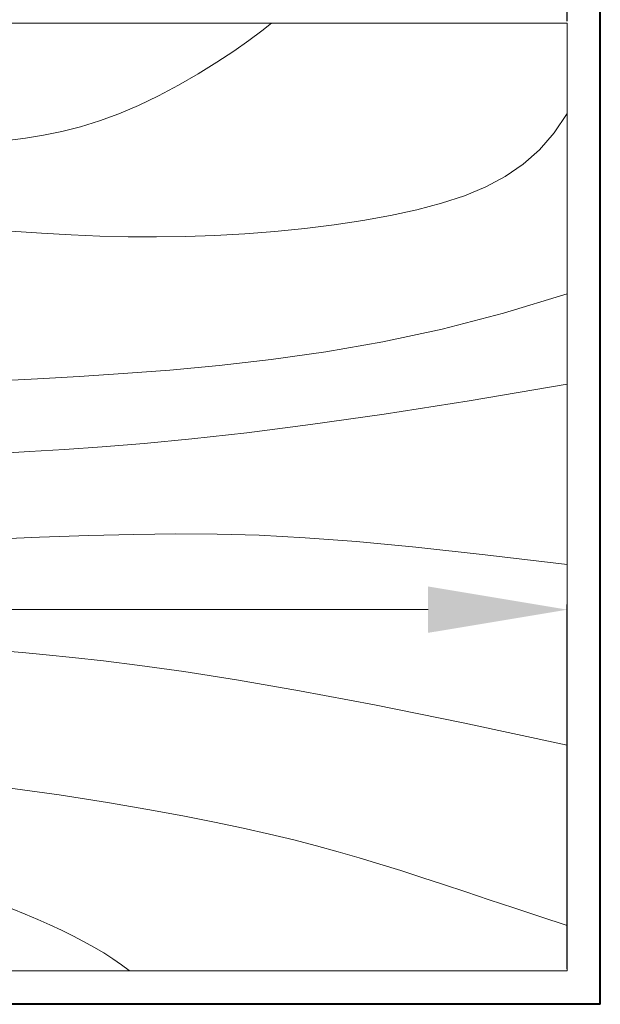
# Model space of a CAD drawing. Units: inches. Extents: x -301 to 715, y -607 to 364.
# Tile 101 of 141: x 103 to 124, y -10 to 26. Entities that reach past the tile are written whole.
import ezdxf

# ---------------------------------------------------------------- set-up
doc = ezdxf.new("R2010")
doc.units = ezdxf.units.IN
doc.header["$MEASUREMENT"] = 0
for name, color, linetype, lineweight in [('A-ANNO-DIMS', 2, 'Continuous', 18), ('A-FURN', 8, 'Continuous', 18), ('A-WALL', 3, 'Continuous', 40)]:
    doc.layers.add(name, color=color, linetype=linetype, lineweight=lineweight)
doc.styles.get("Standard").update_dxf_attribs({"font": 'arial.ttf'})
doc.dimstyles.get("Standard").update_dxf_attribs({"dimtxt": 0.18, "dimasz": 0.18, "dimexe": 0.18, "dimexo": 0.0625, "dimgap": 0.09, "dimtad": 0, "dimtih": 1, "dimtoh": 1, "dimdec": 1, "dimzin": 0, "dimdsep": 46, "dimlunit": 4, "dimtxsty": 'Standard', "dimcen": 0.09, "dimclrd": 3, "dimclre": 4, "dimclrt": 6, "dimadec": 0, "dimazin": 0, "dimtfac": 1, "dimtdec": 1, "dimtofl": 0, "dimtmove": 0, "dimatfit": 3, "dimfxl": 1, "dimtfill": 2, "dimtfillclr": 51, "dimtolj": 1, "dimtzin": 0, "dimarcsym": 0})

# ---------------------------------------------------------------- blocks, each defined once
blk = doc.blocks.new('Table - Square Woodgrain 42 x 42 in.')
blk.add_line((0, -42), (42, -42))
for points in [[(0, -4), (1.704, -4.2172), (3.2358, -4.4188), (4.615, -4.604), (5.8615, -4.7721), (6.9951, -4.9224), (8.0357, -5.0541), (9.0031, -5.1667), (9.9171, -5.2594), (10.7951, -5.3316), (11.6445, -5.3836), (12.4702, -5.4157), (13.277, -5.4283), (14.0698, -5.4217), (14.8535, -5.3964), (15.6331, -5.3526), (16.4133, -5.2908), (17.1986, -5.2103), (17.9913, -5.1062), (18.793, -4.9727), (19.6056, -4.8038), (20.4307, -4.5937), (21.2701, -4.3365), (22.1256, -4.0262), (22.9989, -3.6571), (23.888, -3.2272), (24.7756, -2.7516), (25.6408, -2.2491), (26.4624, -1.7387), (27.2195, -1.2395), (27.891, -0.7703), (28.456, -0.3501), (28.8934, 0.002)], [(0, -42), (0, 0), (42, 0), (42, -42)], [(0, -8), (1.8203, -8.1001), (3.6741, -8.2149), (5.5411, -8.3408), (7.4011, -8.4741), (9.2339, -8.6112), (11.0193, -8.7484), (12.7371, -8.8821), (14.3671, -9.0086), (15.8954, -9.1246), (17.3337, -9.2278), (18.6997, -9.3159), (20.0116, -9.387), (21.2871, -9.4389), (22.5442, -9.4696), (23.8008, -9.477), (25.0749, -9.459), (26.3791, -9.4137), (27.7049, -9.3403), (29.0383, -9.2382), (30.3655, -9.1068), (31.6728, -8.9455), (32.9461, -8.7535), (34.1717, -8.5304), (35.3358, -8.2756), (36.4268, -7.9863), (37.443, -7.6521), (38.3849, -7.2603), (39.253, -6.7986), (40.048, -6.2542), (40.7705, -5.6147), (41.421, -4.8674), (42, -4)], [(42, -12), (39.1784, -12.8621), (36.4519, -13.5654), (33.8246, -14.1294), (31.3004, -14.5731), (28.8832, -14.9161), (26.577, -15.1775), (24.3858, -15.3768), (22.3136, -15.5332), (20.3622, -15.6632), (18.5254, -15.7718), (16.7947, -15.8612), (15.1618, -15.9338), (13.6183, -15.9916), (12.1558, -16.0369), (10.7659, -16.0718), (9.4403, -16.0987), (8.1703, -16.1191), (6.9461, -16.1325), (5.7577, -16.1377), (4.595, -16.1335), (3.4479, -16.1188), (2.3064, -16.0924), (1.1604, -16.0532), (0, -16)], [(42, -16), (37.6529, -16.7365), (33.8802, -17.329), (30.6179, -17.7961), (27.8015, -18.1561), (25.3668, -18.4275), (23.2497, -18.6288), (21.3859, -18.7785), (19.7111, -18.8949), (18.1693, -18.9939), (16.7375, -19.0795), (15.401, -19.1534), (14.1449, -19.217), (12.9544, -19.2717), (11.8148, -19.3191), (10.7113, -19.3606), (9.6291, -19.3976), (8.5534, -19.4323), (7.47, -19.4689), (6.3643, -19.5122), (5.222, -19.5672), (4.0288, -19.6386), (2.7703, -19.7313), (1.4321, -19.8501), (0, -20)], [(0, -24), (3.9243, -23.6805), (7.4766, -23.4138), (10.6891, -23.1954), (13.5943, -23.0205), (16.2247, -22.8847), (18.6125, -22.7832), (20.7903, -22.7116), (22.7903, -22.6651), (24.6563, -22.642), (26.4764, -22.6507), (28.35, -22.7024), (30.3766, -22.8084), (32.6555, -22.98), (35.2861, -23.2283), (38.3678, -23.5645), (42, -24)], [(42, -32), (37.392, -31.017), (33.4585, -30.2231), (30.1291, -29.5949), (27.3334, -29.109), (25.0009, -28.742), (23.0612, -28.4707), (21.4439, -28.2716), (20.0786, -28.1215), (18.8998, -28.0002), (17.8609, -27.9014), (16.9206, -27.8219), (16.0371, -27.7588), (15.1691, -27.709), (14.2748, -27.6693), (13.3128, -27.6368), (12.2415, -27.6083), (11.0295, -27.5824), (9.6867, -27.5643), (8.233, -27.5608), (6.6884, -27.5787), (5.0728, -27.6248), (3.4062, -27.7058), (1.7086, -27.8286), (0, -28)], [(0, -32), (5.4026, -32.5358), (9.9494, -33.019), (13.7424, -33.4553), (16.8834, -33.8505), (19.4743, -34.2106), (21.6171, -34.5413), (23.4136, -34.8486), (24.9657, -35.1382), (26.3614, -35.4156), (27.6332, -35.6841), (28.7995, -35.9467), (29.8788, -36.2064), (30.8897, -36.4661), (31.8507, -36.7288), (32.7802, -36.9973), (33.6968, -37.2747), (34.6175, -37.5635), (35.5531, -37.8651), (36.5128, -38.1805), (37.506, -38.5108), (38.5421, -38.8568), (39.6302, -39.2197), (40.7797, -39.6004), (42, -40)], [(0, -36), (3.0098, -36.2857), (5.5354, -36.5643), (7.6368, -36.8359), (9.374, -37.1009), (10.807, -37.3597), (11.9957, -37.6126), (13.0002, -37.8599), (13.8804, -38.102), (14.6874, -38.3393), (15.4365, -38.5729), (16.1338, -38.8041), (16.7858, -39.0341), (17.3987, -39.264), (17.9787, -39.4952), (18.5322, -39.7288), (19.0655, -39.9662), (19.5832, -40.2081), (20.0842, -40.4544), (20.5657, -40.7046), (21.0249, -40.9581), (21.459, -41.2144), (21.8653, -41.4731), (22.2409, -41.7335), (22.5831, -41.9951)]]:
    blk.add_lwpolyline(points)
blk = doc.blocks.new('*D48')
at = {"layer": 'A-ANNO-DIMS', "color": 0, "lineweight": -2, "transparency": 16777216}
for p, q in [((-45.603, -7.657), (-45.603, 4.543)), ((122.71, -8.548), (122.71, 4.543))]:
    blk.add_line(p, q, dxfattribs=at)
at = {"layer": 'A-ANNO-DIMS', "color": 0, "lineweight": 0, "transparency": 16777216}
for p, q in [((-40.603, 4.363), (32.358, 4.363)), ((117.71, 4.363), (44.749, 4.363))]:
    blk.add_line(p, q, dxfattribs=at)
at = {"layer": 'A-ANNO-DIMS', "color": 0, "transparency": 16777216}
for points in [[(-40.603, 5.197), (-40.603, 3.53), (-45.603, 4.363)], [(117.71, 5.197), (117.71, 3.53), (122.71, 4.363)]]:
    blk.add_solid(points, dxfattribs=at)
at = {"layer": 'Defpoints', "color": 0, "transparency": 16777216}
for p in [(-45.603, 4.363), (-45.603, -7.72), (122.71, -8.61)]:
    blk.add_point(p, dxfattribs=at)
at = {"layer": 'A-ANNO-DIMS', "color": 0, "transparency": 16777216, "insert": (38.553, 4.363), "char_height": 3, "attachment_point": 5, "bg_fill": 1, "box_fill_scale": 1.25, "bg_fill_color": 51, "bg_fill_transparency": 0}
blk.add_mtext('\\A1;14\'-0{\\H1x;\\S1/2;}"', dxfattribs=at)
blk = doc.blocks.new('*D119')
at = {"layer": 'A-ANNO-DIMS', "color": 4, "lineweight": -2, "transparency": 16777216}
for p, q in [((88.66, 25.504), (88.66, 30.729)), ((122.71, 25.504), (122.71, 30.729))]:
    blk.add_line(p, q, dxfattribs=at)
at = {"layer": 'A-ANNO-DIMS', "color": 3, "lineweight": -2, "transparency": 16777216}
for p, q in [((88.84, 30.549), (104.975, 30.549)), ((122.53, 30.549), (106.395, 30.549))]:
    blk.add_line(p, q, dxfattribs=at)
at = {"layer": 'A-ANNO-DIMS', "color": 3, "transparency": 16777216}
for points in [[(88.84, 30.579), (88.84, 30.519), (88.66, 30.549)], [(122.53, 30.579), (122.53, 30.519), (122.71, 30.549)]]:
    blk.add_solid(points, dxfattribs=at)
at = {"layer": 'Defpoints', "color": 0, "transparency": 16777216}
for p in [(122.71, 30.549), (88.66, 25.442), (122.71, 25.442)]:
    blk.add_point(p, dxfattribs=at)
at = {"layer": 'A-ANNO-DIMS', "color": 6, "transparency": 16777216, "insert": (105.685, 30.549), "char_height": 0.18, "attachment_point": 5, "bg_fill": 1, "box_fill_scale": 1.25, "bg_fill_color": 51, "bg_fill_transparency": 0}
blk.add_mtext('\\A1;2\'-10" TYP.', dxfattribs=at)

msp = doc.modelspace()

# ---------------------------------------------------------------- linework, layer by layer
at = {"layer": 'A-WALL'}
for q in [(123.897, 193.182), (21.897, -9.818)]:
    msp.add_line((123.897, -9.818), q, dxfattribs=at)

# ---------------------------------------------------------------- block references
at = {"layer": 'A-FURN', "xscale": 0.8107193059798699, "yscale": 0.8107193059798699, "zscale": 0.8107193059798699}
msp.add_blockref('Table - Square Woodgrain 42 x 42 in.', (88.66, 25.44), dxfattribs=at)

# ---------------------------------------------------------------- dimensions: what is measured, and where the dimension line sits
at = {"layer": 'A-ANNO-DIMS'}
dim = msp.add_linear_dim(base=(122.7099, 30.5493), p1=(88.6597, 25.4415), p2=(122.7099, 25.4415), text='<> TYP.', dimstyle='Standard', override={"dimdec": 1, "dimlfac": 1, "dimrnd": 0, "dimzin": 1, "dimdsep": 46, "dimlunit": 4, "dimfrac": 2}, dxfattribs=at)
dim.commit()
dim.dimension.update_dxf_attribs({"geometry": '*D119', "text_midpoint": (105.6848, 30.5493)})
dim = msp.add_linear_dim(base=(-45.603, 4.363), p1=(122.71, -8.61), p2=(-45.603, -7.72), dimstyle='Standard', override={"dimtxt": 3, "dimasz": 5, "dimclrd": 0, "dimclre": 0, "dimclrt": 0, "dimlwd": 0}, dxfattribs=at)
dim.commit()
dim.dimension.update_dxf_attribs({"geometry": '*D48', "text_midpoint": (38.553, 4.363)})

doc.saveas('drawing.dxf')
